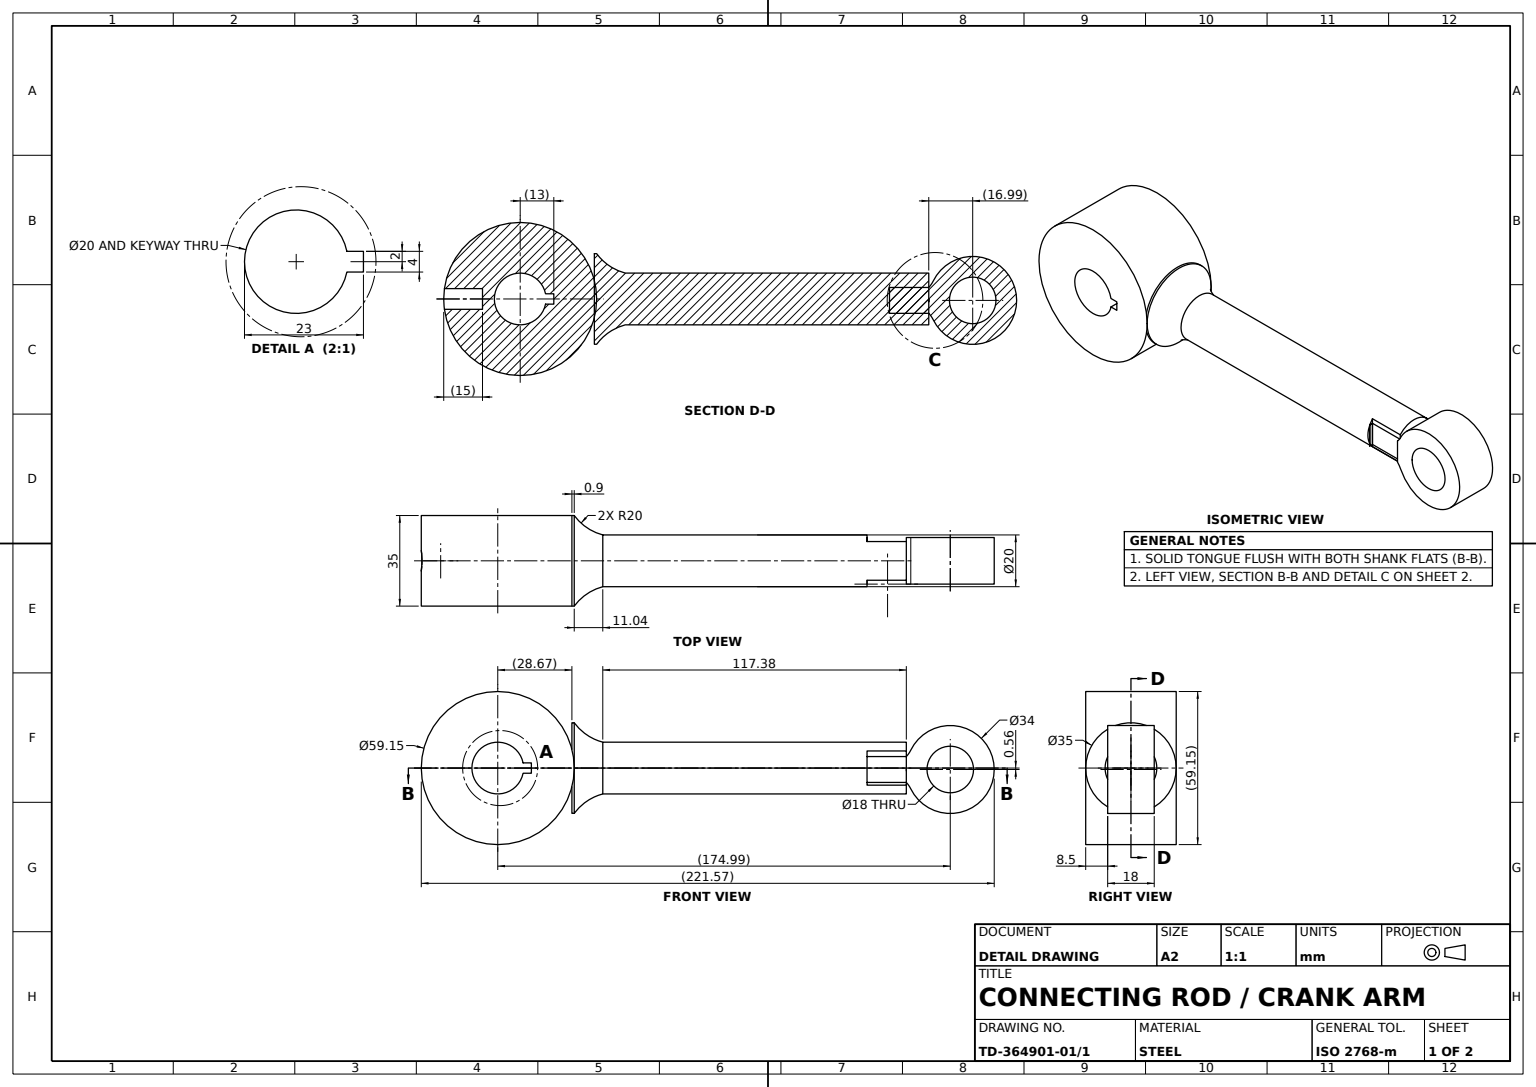
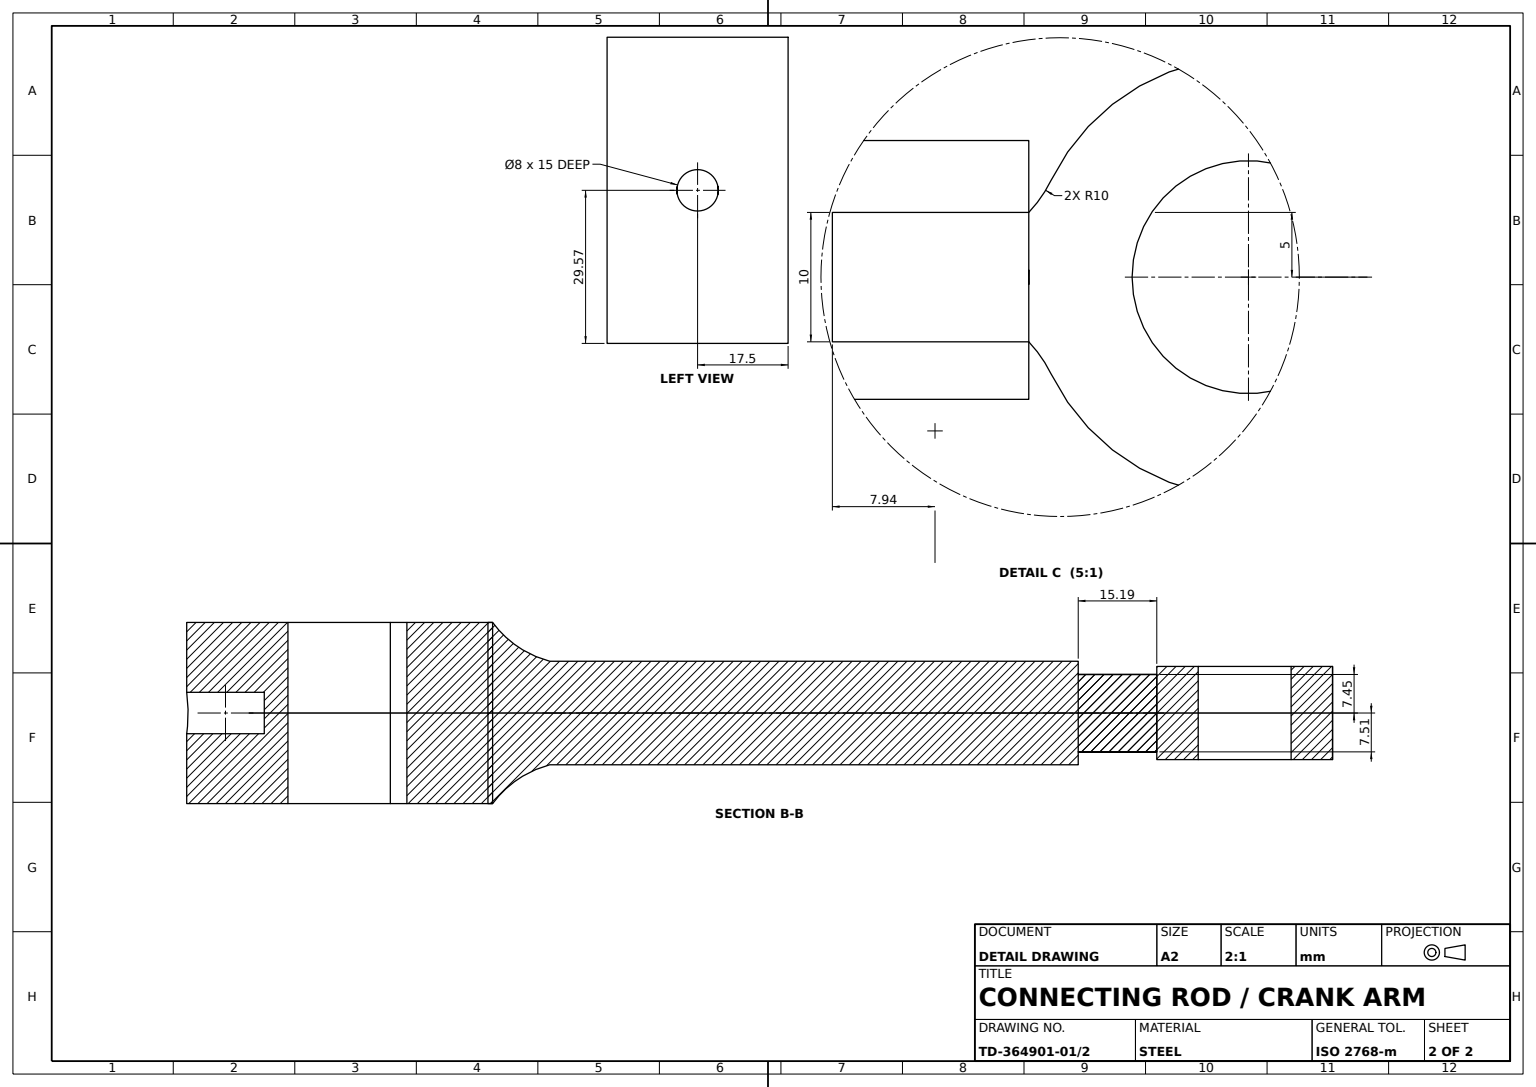
SolidWorks part; units mm, degrees
material "Plain Carbon Steel"
ref_plane "Front Plane" through (0, 0, 0) normal (0, 0, 1) x (1, 0, 0)
ref_plane "Top Plane" through (0, 0, 0) normal (0, 1, 0) x (1, 0, 0)
ref_plane "Right Plane" through (0, 0, 0) normal (1, 0, 0) x (0, 0, -1)
sketch "Rod Shank Profile" plane through (0, 0, 0) normal (0, 0, 1) x (1, 0, 0)
  line L0 (0, 0) -> (25, 0) construction
  line L1 (-10, 0) -> (13, 0) construction
  line L2 (34.617, 10) -> (152, 10)
  line L3 (152, 10) -> (152, 0)
  line L4 (34.617, 0) -> (152, 0)
  line L5 (34.617, 10) -> (34.617, 0)
  line L6 (34.617, 0) -> (152, 0) construction
  circle A0 centre (0, 0) radius 10
  dimension "D1" = 20
  dimension "D2" = 10
  dimension "D3" = 23
  dimension "D4" = 152
  dimension "D5" = 25
  dimension "D6" = 117.383
revolve "Rod Shank" add sketch "Rod Shank Profile" angle 360 about L0
sketch "Big End Eye Profile" plane through (0, 0, 0) normal (0, 0, 1) x (1, 0, 0)
  line L1 (7, -2) -> (7, 2)
  line L2 (3.798, -2) -> (7, -2)
  line L3 (3.798, 2) -> (7, 2)
  line L4 (-16, 0) -> (-14.4771, 0) construction
  line L7 (19, 15.9732) -> (19, 15.8005)
  line L8 (19, -15.8005) -> (19, -15.9732)
  circle A0 centre (-6, 0) radius 29.5746
  arc A1 (3.798, 2) -> (3.798, -2) centre (-6, 0) ccw
  dimension "D1" = 20
  dimension "D4" = 12
  dimension "D2" = 59.1492
  dimension "D5" = 15.202
  dimension "D3" = 6
  dimension "D6" = 25
  dimension "D7" = 17.9732
extrude "Big End Eye" add sketch "Big End Eye Profile" along normal mid plane 35 contours A0 A1 L3 L1 L2
sketch "Small End Eye Profile" plane through (0, 0, 0) normal (0, 0, 1) x (1, 0, 0)
  line L0 (168.9909, -0.5555) -> (136.8082, -0.5555) construction
  line L1 (152, -5.5555) -> (136.8082, -5.5555)
  line L2 (152, 10) -> (152, -10)
  line L3 (168.9909, -5.5555) -> (161.5076, -5.5555)
  line L4 (152, 4.4445) -> (136.8082, 4.4445)
  line L5 (168.9909, -5.5555) -> (136.8082, -5.5555) construction
  line L6 (136.8082, -5.5555) -> (136.8082, 4.4445)
  circle A0 centre (168.9909, -0.5555) radius 9
  arc A1 (152, 0) -> (152, -1.111) centre (168.9909, -0.5555) ccw
  arc A2 (152, -5.5555) -> (153.7264, -8.0384) centre (144.7472, -12.4401) cw
  arc A3 (152, 4.4445) -> (153.7264, 6.9274) centre (144.7472, 11.329) ccw
  arc A4 (153.7264, -8.0384) -> (153.7264, 6.9274) centre (168.9909, -0.5555) ccw
  point P0 (152, 0)
  dimension "D2" = 34
  dimension "D3" = 18
  dimension "D1" = 10
  dimension "D4" = 7.9391
  dimension "D5" = 15.1918
  dimension "D6" = 5
extrude "Small End Eye" add sketch "Small End Eye Profile" along normal mid plane 18 contours A2 A4 A3 L2 A0 | A1 L2 L4 L6 L1
sketch "Big End Neck Profile" plane through (0, 0, 0) normal (0, 1, 0) x (1, 0, 0)
  line L0 (34.617, 10) -> (34.617, 0)
  line L1 (34.617, 10) -> (34.617, -10) construction
  line L2 (34.617, 0) -> (23.5746, 0)
  line L3 (23.5746, -17.5) -> (23.5746, 17.5) construction
  line L9 (23.5746, 17.5) -> (22.6732, 17.5)
  line L10 (23.5746, 17.5) -> (-35.5746, 17.5) construction
  line L11 (22.6732, 17.5) -> (22.6732, 0)
  line L12 (22.6732, 0) -> (23.5746, 0)
  arc A0 (34.617, 10) -> (23.5746, 17.5) centre (39.6887, 29.3463) cw
  dimension "D1" = 20
  dimension "D2" = 0.9013
revolve "Big End Neck" add sketch "Big End Neck Profile" angle 360 about L2
sketch "Small End Flat Profile" plane through (0, 0, 0) normal (0, 1, 0) x (1, 0, 0)
  line L0 (152, -10) -> (152, 10) construction
  line L1 (152, -7.5057) -> (136.8084, -7.5057)
  line L2 (152, -7.5057) -> (152, -13.3883)
  line L3 (152, -13.3883) -> (136.8084, -13.3883)
  line L4 (136.8084, -7.5057) -> (136.8084, -13.3883)
  line L6 (152, 7.4458) -> (136.8084, 7.4458)
  line L7 (152, 7.4458) -> (152, 16.0246)
  line L8 (152, 16.0246) -> (136.8084, 16.0246)
  line L9 (136.8084, 7.4458) -> (136.8084, 16.0246)
  dimension "D1" = 15.1916
  dimension "D2" = 7.5057
  dimension "D3" = 5.8826
  dimension "D4" = 7.4458
  dimension "D5" = 8.5787
extrude "Small End Flat Cut" cut sketch "Small End Flat Profile" against normal through all both and the other way through all
sketch "Big End Hub Profile" plane through (0, 0, 0) normal (0, 1, 0) x (1, 0, 0)
  line L0 (-20.5746, 0) -> (-35.5746, 0) construction
  line L1 (-35.5746, 17.5) -> (-35.5746, -17.5) construction
  line L2 (-20.5746, 4) -> (-35.5746, 4)
  line L3 (-35.5746, 0) -> (-20.5746, 0)
  line L4 (-20.5746, 4) -> (-20.5746, 0)
  line L5 (0, 4) -> (-35.5746, 4) construction
  line L6 (0, 0) -> (-35.5746, 0) construction
  line L8 (-35.5746, 0) -> (-35.5746, 4)
  dimension "D3" = 15
  dimension "D1" = 4
revolve "Big End Hub" add sketch "Big End Hub Profile" angle 360 about L3
sketch "Big End Keyway Profile" plane through (-35.5746, 0, 0) normal (-1, 0, 0) x (0, 0, 1)
  circle A0 centre (0, 0) radius 4
  dimension "D1" = 8
extrude "Big End Keyway Cut" cut sketch "Big End Keyway Profile" against normal blind 15
